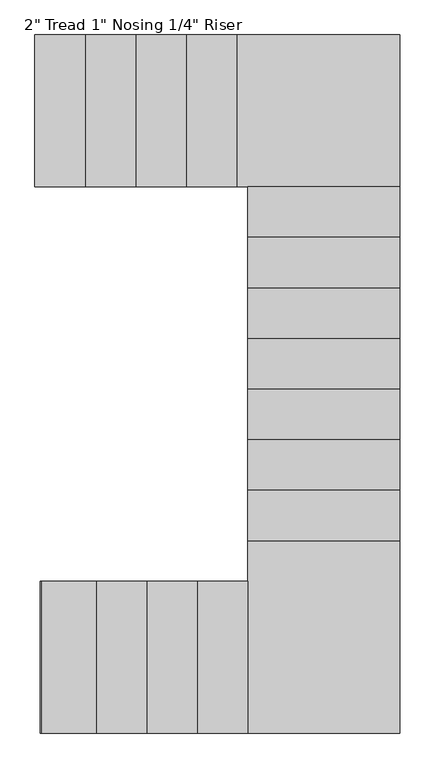
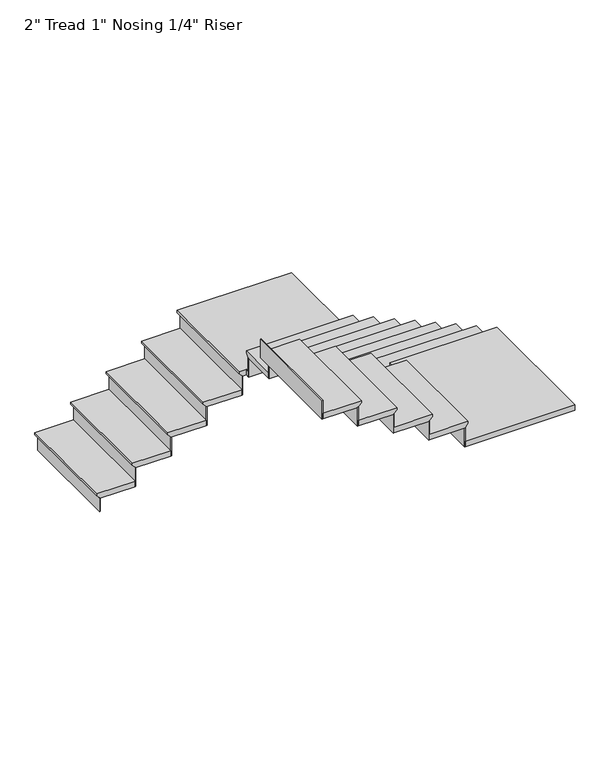
"""IFC4 building model written with IfcOpenShell, lengths in millimetres: stair flight geometry."""

from ifc_helpers import new_model, si_unit, origin, place, context, project, spatial, faceted_brep, source, transform, mapped, element, save


def stair_flight_4d0103da(model_context):
    return source(origin(), model_context, "Body", "Brep", [
        faceted_brep([(-11350.6229553, 1140.6964313, 455.0833333), (-11350.6229553, 1140.6964313, 474.1333333), (-11350.6229553, 2055.0964313, 474.1333333), (-11350.6229553, 2055.0964313, 455.0833333), (-11325.2229553, 1140.6964313, 429.6833333), (-11325.2229553, 2055.0964313, 429.6833333), (-11020.4229553, 1140.6964313, 474.1333333), (-11020.4229553, 2055.0964313, 474.1333333), (-11325.2229553, 2055.0964313, 423.3333333), (-11020.4229553, 2055.0964313, 423.3333333), (-11020.4229553, 1140.6964313, 423.3333333), (-11325.2229553, 1140.6964313, 423.3333333)], [[[0, 1, 2, 3]], [[4, 0, 3, 5]], [[2, 1, 6, 7]], [[8, 9, 10, 11]], [[2, 7, 9, 8, 5, 3]], [[8, 11, 4, 5]], [[6, 1, 0, 4, 11, 10]], [[7, 6, 10, 9]]]),
        faceted_brep([(-11325.2229553, 1140.6964313, 423.3333333), (-11325.2229553, 1140.6964313, 304.8), (-11318.8729553, 1140.6964313, 304.8), (-11318.8729553, 1140.6964313, 423.3333333), (-11325.2229553, 2055.0964313, 423.3333333), (-11318.8729553, 2055.0964313, 423.3333333), (-11318.8729553, 2055.0964313, 304.8), (-11325.2229553, 2055.0964313, 304.8)], [[[0, 1, 2, 3]], [[4, 5, 6, 7]], [[1, 0, 4, 7]], [[2, 1, 7, 6]], [[3, 2, 6, 5]], [[0, 3, 5, 4]]]),
        faceted_brep([(-11020.4229553, 1140.6964313, 592.6666667), (-11020.4229553, 1140.6964313, 423.3333333), (-11014.0729553, 1140.6964313, 423.3333333), (-11014.0729553, 1140.6964313, 592.6666667), (-11020.4229553, 2055.0964313, 592.6666667), (-11014.0729553, 2055.0964313, 592.6666667), (-11014.0729553, 2055.0964313, 423.3333333), (-11020.4229553, 2055.0964313, 423.3333333)], [[[0, 1, 2, 3]], [[4, 5, 6, 7]], [[1, 0, 4, 7]], [[2, 1, 7, 6]], [[3, 2, 6, 5]], [[0, 3, 5, 4]]]),
        faceted_brep([(-11045.8229553, 2055.0964313, 643.4666667), (-11045.8229553, 1140.6964313, 643.4666667), (-10715.6229553, 1140.6964313, 643.4666667), (-10715.6229553, 2055.0964313, 643.4666667), (-11020.4229553, 2055.0964313, 592.6666667), (-10715.6229553, 2055.0964313, 592.6666667), (-10715.6229553, 1140.6964313, 592.6666667), (-11020.4229553, 1140.6964313, 592.6666667), (-11020.4229553, 2055.0964313, 599.0166667), (-11045.8229553, 2055.0964313, 624.4166667), (-11020.4229553, 1140.6964313, 599.0166667), (-11045.8229553, 1140.6964313, 624.4166667)], [[[0, 1, 2, 3]], [[4, 5, 6, 7]], [[0, 3, 5, 4, 8, 9]], [[4, 7, 10, 8]], [[2, 1, 11, 10, 7, 6]], [[3, 2, 6, 5]], [[11, 1, 0, 9]], [[10, 11, 9, 8]]]),
        faceted_brep([(-10715.6229553, 1140.6964313, 762.0), (-10715.6229553, 1140.6964313, 592.6666667), (-10709.2729553, 1140.6964313, 592.6666667), (-10709.2729553, 1140.6964313, 762.0), (-10715.6229553, 2055.0964313, 762.0), (-10709.2729553, 2055.0964313, 762.0), (-10709.2729553, 2055.0964313, 592.6666667), (-10715.6229553, 2055.0964313, 592.6666667)], [[[0, 1, 2, 3]], [[4, 5, 6, 7]], [[1, 0, 4, 7]], [[2, 1, 7, 6]], [[3, 2, 6, 5]], [[0, 3, 5, 4]]]),
        faceted_brep([(-10741.0229553, 2055.0964313, 812.8), (-10741.0229553, 1140.6964313, 812.8), (-10410.8229553, 1140.6964313, 812.8), (-10410.8229553, 2055.0964313, 812.8), (-10715.6229553, 2055.0964313, 762.0), (-10410.8229553, 2055.0964313, 762.0), (-10410.8229553, 1140.6964313, 762.0), (-10715.6229553, 1140.6964313, 762.0), (-10715.6229553, 2055.0964313, 768.35), (-10741.0229553, 2055.0964313, 793.75), (-10715.6229553, 1140.6964313, 768.35), (-10741.0229553, 1140.6964313, 793.75)], [[[0, 1, 2, 3]], [[4, 5, 6, 7]], [[0, 3, 5, 4, 8, 9]], [[4, 7, 10, 8]], [[2, 1, 11, 10, 7, 6]], [[3, 2, 6, 5]], [[11, 1, 0, 9]], [[10, 11, 9, 8]]]),
        faceted_brep([(-10410.8229553, 1140.6964313, 931.3333333), (-10410.8229553, 1140.6964313, 762.0), (-10404.4729553, 1140.6964313, 762.0), (-10404.4729553, 1140.6964313, 931.3333333), (-10410.8229553, 2055.0964313, 931.3333333), (-10404.4729553, 2055.0964313, 931.3333333), (-10404.4729553, 2055.0964313, 762.0), (-10410.8229553, 2055.0964313, 762.0)], [[[0, 1, 2, 3]], [[4, 5, 6, 7]], [[1, 0, 4, 7]], [[2, 1, 7, 6]], [[3, 2, 6, 5]], [[0, 3, 5, 4]]]),
        faceted_brep([(-10436.2229553, 2055.0964313, 982.1333333), (-10436.2229553, 1140.6964313, 982.1333333), (-10106.0229553, 1140.6964313, 982.1333333), (-10106.0229553, 2055.0964313, 982.1333333), (-10410.8229553, 2055.0964313, 931.3333333), (-10106.0229553, 2055.0964313, 931.3333333), (-10106.0229553, 1140.6964313, 931.3333333), (-10410.8229553, 1140.6964313, 931.3333333), (-10410.8229553, 2055.0964313, 937.6833333), (-10436.2229553, 2055.0964313, 963.0833333), (-10410.8229553, 1140.6964313, 937.6833333), (-10436.2229553, 1140.6964313, 963.0833333)], [[[0, 1, 2, 3]], [[4, 5, 6, 7]], [[0, 3, 5, 4, 8, 9]], [[4, 7, 10, 8]], [[2, 1, 11, 10, 7, 6]], [[3, 2, 6, 5]], [[11, 1, 0, 9]], [[10, 11, 9, 8]]]),
        faceted_brep([(-10106.0229553, 1140.6964313, 1100.6666667), (-10106.0229553, 1140.6964313, 931.3333333), (-10099.6729553, 1140.6964313, 931.3333333), (-10099.6729553, 1140.6964313, 1100.6666667), (-10106.0229553, 2055.0964313, 1100.6666667), (-10099.6729553, 2055.0964313, 1100.6666667), (-10099.6729553, 2055.0964313, 931.3333333), (-10106.0229553, 2055.0964313, 931.3333333)], [[[0, 1, 2, 3]], [[4, 5, 6, 7]], [[1, 0, 4, 7]], [[2, 1, 7, 6]], [[3, 2, 6, 5]], [[0, 3, 5, 4]]]),
        faceted_brep([(-9153.5229553, 1115.2964313, 1151.4666667), (-9153.5229553, 2055.0964313, 1151.4666667), (-10131.4229553, 2055.0964313, 1151.4666667), (-10131.4229553, 1140.6964313, 1151.4666667), (-10067.9229553, 1140.6964313, 1151.4666667), (-10067.9229553, 1115.2964313, 1151.4666667), (-9153.5229553, 2055.0964313, 1100.6666667), (-9153.5229553, 1115.2964313, 1100.6666667), (-10067.9229553, 1115.2964313, 1100.6666667), (-10067.9229553, 1140.6964313, 1100.6666667), (-10106.0229553, 1140.6964313, 1100.6666667), (-10106.0229553, 2055.0964313, 1100.6666667), (-10106.0229553, 2055.0964313, 1107.0166667), (-10131.4229553, 2055.0964313, 1132.4166667), (-10106.0229553, 1140.6964313, 1107.0166667), (-10131.4229553, 1140.6964313, 1132.4166667)], [[[0, 1, 2, 3, 4, 5]], [[6, 7, 8, 9, 10, 11]], [[1, 0, 7, 6]], [[2, 1, 6, 11, 12, 13]], [[11, 10, 14, 12]], [[4, 3, 15, 14, 10, 9]], [[5, 4, 9, 8]], [[0, 5, 8, 7]], [[15, 3, 2, 13]], [[14, 15, 13, 12]]]),
        faceted_brep([(-10067.9229553, 1115.2964313, 1270.0), (-10067.9229553, 1115.2964313, 1100.6666667), (-10067.9229553, 1108.9464313, 1100.6666667), (-10067.9229553, 1108.9464313, 1270.0), (-9153.5229553, 1115.2964313, 1270.0), (-9153.5229553, 1108.9464313, 1270.0), (-9153.5229553, 1108.9464313, 1100.6666667), (-9153.5229553, 1115.2964313, 1100.6666667)], [[[0, 1, 2, 3]], [[4, 5, 6, 7]], [[1, 0, 4, 7]], [[2, 1, 7, 6]], [[3, 2, 6, 5]], [[0, 3, 5, 4]]]),
        faceted_brep([(-9153.5229553, 1140.6964313, 1320.8), (-10067.9229553, 1140.6964313, 1320.8), (-10067.9229553, 810.4964313, 1320.8), (-9153.5229553, 810.4964313, 1320.8), (-9153.5229553, 1115.2964313, 1270.0), (-9153.5229553, 810.4964313, 1270.0), (-10067.9229553, 810.4964313, 1270.0), (-10067.9229553, 1115.2964313, 1270.0), (-9153.5229553, 1115.2964313, 1276.35), (-9153.5229553, 1140.6964313, 1301.75), (-10067.9229553, 1115.2964313, 1276.35), (-10067.9229553, 1140.6964313, 1301.75)], [[[0, 1, 2, 3]], [[4, 5, 6, 7]], [[0, 3, 5, 4, 8, 9]], [[4, 7, 10, 8]], [[2, 1, 11, 10, 7, 6]], [[3, 2, 6, 5]], [[11, 1, 0, 9]], [[10, 11, 9, 8]]]),
        faceted_brep([(-10067.9229553, 810.4964313, 1439.3333333), (-10067.9229553, 810.4964313, 1270.0), (-10067.9229553, 804.1464313, 1270.0), (-10067.9229553, 804.1464313, 1439.3333333), (-9153.5229553, 810.4964313, 1439.3333333), (-9153.5229553, 804.1464313, 1439.3333333), (-9153.5229553, 804.1464313, 1270.0), (-9153.5229553, 810.4964313, 1270.0)], [[[0, 1, 2, 3]], [[4, 5, 6, 7]], [[1, 0, 4, 7]], [[2, 1, 7, 6]], [[3, 2, 6, 5]], [[0, 3, 5, 4]]]),
        faceted_brep([(-9153.5229553, 835.8964313, 1490.1333333), (-10067.9229553, 835.8964313, 1490.1333333), (-10067.9229553, 505.6964313, 1490.1333333), (-9153.5229553, 505.6964313, 1490.1333333), (-9153.5229553, 810.4964313, 1439.3333333), (-9153.5229553, 505.6964313, 1439.3333333), (-10067.9229553, 505.6964313, 1439.3333333), (-10067.9229553, 810.4964313, 1439.3333333), (-9153.5229553, 810.4964313, 1445.6833333), (-9153.5229553, 835.8964313, 1471.0833333), (-10067.9229553, 810.4964313, 1445.6833333), (-10067.9229553, 835.8964313, 1471.0833333)], [[[0, 1, 2, 3]], [[4, 5, 6, 7]], [[0, 3, 5, 4, 8, 9]], [[4, 7, 10, 8]], [[2, 1, 11, 10, 7, 6]], [[3, 2, 6, 5]], [[11, 1, 0, 9]], [[10, 11, 9, 8]]]),
        faceted_brep([(-10067.9229553, 505.6964313, 1608.6666667), (-10067.9229553, 505.6964313, 1439.3333333), (-10067.9229553, 499.3464313, 1439.3333333), (-10067.9229553, 499.3464313, 1608.6666667), (-9153.5229553, 505.6964313, 1608.6666667), (-9153.5229553, 499.3464313, 1608.6666667), (-9153.5229553, 499.3464313, 1439.3333333), (-9153.5229553, 505.6964313, 1439.3333333)], [[[0, 1, 2, 3]], [[4, 5, 6, 7]], [[1, 0, 4, 7]], [[2, 1, 7, 6]], [[3, 2, 6, 5]], [[0, 3, 5, 4]]]),
        faceted_brep([(-9153.5229553, 531.0964313, 1659.4666667), (-10067.9229553, 531.0964313, 1659.4666667), (-10067.9229553, 200.8964313, 1659.4666667), (-9153.5229553, 200.8964313, 1659.4666667), (-9153.5229553, 505.6964313, 1608.6666667), (-9153.5229553, 200.8964313, 1608.6666667), (-10067.9229553, 200.8964313, 1608.6666667), (-10067.9229553, 505.6964313, 1608.6666667), (-9153.5229553, 505.6964313, 1615.0166667), (-9153.5229553, 531.0964313, 1640.4166667), (-10067.9229553, 505.6964313, 1615.0166667), (-10067.9229553, 531.0964313, 1640.4166667)], [[[0, 1, 2, 3]], [[4, 5, 6, 7]], [[0, 3, 5, 4, 8, 9]], [[4, 7, 10, 8]], [[2, 1, 11, 10, 7, 6]], [[3, 2, 6, 5]], [[11, 1, 0, 9]], [[10, 11, 9, 8]]]),
        faceted_brep([(-10067.9229553, 200.8964313, 1778.0), (-10067.9229553, 200.8964313, 1608.6666667), (-10067.9229553, 194.5464313, 1608.6666667), (-10067.9229553, 194.5464313, 1778.0), (-9153.5229553, 200.8964313, 1778.0), (-9153.5229553, 194.5464313, 1778.0), (-9153.5229553, 194.5464313, 1608.6666667), (-9153.5229553, 200.8964313, 1608.6666667)], [[[0, 1, 2, 3]], [[4, 5, 6, 7]], [[1, 0, 4, 7]], [[2, 1, 7, 6]], [[3, 2, 6, 5]], [[0, 3, 5, 4]]]),
        faceted_brep([(-9153.5229553, 226.2964313, 1828.8), (-10067.9229553, 226.2964313, 1828.8), (-10067.9229553, -103.9035687, 1828.8), (-9153.5229553, -103.9035687, 1828.8), (-9153.5229553, 200.8964313, 1778.0), (-9153.5229553, -103.9035687, 1778.0), (-10067.9229553, -103.9035687, 1778.0), (-10067.9229553, 200.8964313, 1778.0), (-9153.5229553, 200.8964313, 1784.35), (-9153.5229553, 226.2964313, 1809.75), (-10067.9229553, 200.8964313, 1784.35), (-10067.9229553, 226.2964313, 1809.75)], [[[0, 1, 2, 3]], [[4, 5, 6, 7]], [[0, 3, 5, 4, 8, 9]], [[4, 7, 10, 8]], [[2, 1, 11, 10, 7, 6]], [[3, 2, 6, 5]], [[11, 1, 0, 9]], [[10, 11, 9, 8]]]),
        faceted_brep([(-10067.9229553, -103.9035687, 1947.3333333), (-10067.9229553, -103.9035687, 1778.0), (-10067.9229553, -110.2535687, 1778.0), (-10067.9229553, -110.2535687, 1947.3333333), (-9153.5229553, -103.9035687, 1947.3333333), (-9153.5229553, -110.2535687, 1947.3333333), (-9153.5229553, -110.2535687, 1778.0), (-9153.5229553, -103.9035687, 1778.0)], [[[0, 1, 2, 3]], [[4, 5, 6, 7]], [[1, 0, 4, 7]], [[2, 1, 7, 6]], [[3, 2, 6, 5]], [[0, 3, 5, 4]]]),
        faceted_brep([(-9153.5229553, -78.5035687, 1998.1333333), (-10067.9229553, -78.5035687, 1998.1333333), (-10067.9229553, -408.7035687, 1998.1333333), (-9153.5229553, -408.7035687, 1998.1333333), (-9153.5229553, -103.9035687, 1947.3333333), (-9153.5229553, -408.7035687, 1947.3333333), (-10067.9229553, -408.7035687, 1947.3333333), (-10067.9229553, -103.9035687, 1947.3333333), (-9153.5229553, -103.9035687, 1953.6833333), (-9153.5229553, -78.5035687, 1979.0833333), (-10067.9229553, -103.9035687, 1953.6833333), (-10067.9229553, -78.5035687, 1979.0833333)], [[[0, 1, 2, 3]], [[4, 5, 6, 7]], [[0, 3, 5, 4, 8, 9]], [[4, 7, 10, 8]], [[2, 1, 11, 10, 7, 6]], [[3, 2, 6, 5]], [[11, 1, 0, 9]], [[10, 11, 9, 8]]]),
        faceted_brep([(-10067.9229553, -408.7035687, 2116.6666667), (-10067.9229553, -408.7035687, 1947.3333333), (-10067.9229553, -415.0535687, 1947.3333333), (-10067.9229553, -415.0535687, 2116.6666667), (-9153.5229553, -408.7035687, 2116.6666667), (-9153.5229553, -415.0535687, 2116.6666667), (-9153.5229553, -415.0535687, 1947.3333333), (-9153.5229553, -408.7035687, 1947.3333333)], [[[0, 1, 2, 3]], [[4, 5, 6, 7]], [[1, 0, 4, 7]], [[2, 1, 7, 6]], [[3, 2, 6, 5]], [[0, 3, 5, 4]]]),
        faceted_brep([(-9153.5229553, -383.3035687, 2167.4666667), (-10067.9229553, -383.3035687, 2167.4666667), (-10067.9229553, -713.5035687, 2167.4666667), (-9153.5229553, -713.5035687, 2167.4666667), (-9153.5229553, -408.7035687, 2116.6666667), (-9153.5229553, -713.5035687, 2116.6666667), (-10067.9229553, -713.5035687, 2116.6666667), (-10067.9229553, -408.7035687, 2116.6666667), (-9153.5229553, -408.7035687, 2123.0166667), (-9153.5229553, -383.3035687, 2148.4166667), (-10067.9229553, -408.7035687, 2123.0166667), (-10067.9229553, -383.3035687, 2148.4166667)], [[[0, 1, 2, 3]], [[4, 5, 6, 7]], [[0, 3, 5, 4, 8, 9]], [[4, 7, 10, 8]], [[2, 1, 11, 10, 7, 6]], [[3, 2, 6, 5]], [[11, 1, 0, 9]], [[10, 11, 9, 8]]]),
        faceted_brep([(-10067.9229553, -713.5035687, 2286.0), (-10067.9229553, -713.5035687, 2116.6666667), (-10067.9229553, -719.8535687, 2116.6666667), (-10067.9229553, -719.8535687, 2286.0), (-9153.5229553, -713.5035687, 2286.0), (-9153.5229553, -719.8535687, 2286.0), (-9153.5229553, -719.8535687, 2116.6666667), (-9153.5229553, -713.5035687, 2116.6666667)], [[[0, 1, 2, 3]], [[4, 5, 6, 7]], [[1, 0, 4, 7]], [[2, 1, 7, 6]], [[3, 2, 6, 5]], [[0, 3, 5, 4]]]),
        faceted_brep([(-9153.5229553, -688.1035687, 2336.8), (-10067.9229553, -688.1035687, 2336.8), (-10067.9229553, -1018.3035687, 2336.8), (-9153.5229553, -1018.3035687, 2336.8), (-9153.5229553, -713.5035687, 2286.0), (-9153.5229553, -1018.3035687, 2286.0), (-10067.9229553, -1018.3035687, 2286.0), (-10067.9229553, -713.5035687, 2286.0), (-9153.5229553, -713.5035687, 2292.35), (-9153.5229553, -688.1035687, 2317.75), (-10067.9229553, -713.5035687, 2292.35), (-10067.9229553, -688.1035687, 2317.75)], [[[0, 1, 2, 3]], [[4, 5, 6, 7]], [[0, 3, 5, 4, 8, 9]], [[4, 7, 10, 8]], [[2, 1, 11, 10, 7, 6]], [[3, 2, 6, 5]], [[11, 1, 0, 9]], [[10, 11, 9, 8]]]),
        faceted_brep([(-10067.9229553, -1018.3035687, 2455.3333333), (-10067.9229553, -1018.3035687, 2286.0), (-10067.9229553, -1024.6535687, 2286.0), (-10067.9229553, -1024.6535687, 2455.3333333), (-9153.5229553, -1018.3035687, 2455.3333333), (-9153.5229553, -1024.6535687, 2455.3333333), (-9153.5229553, -1024.6535687, 2286.0), (-9153.5229553, -1018.3035687, 2286.0)], [[[0, 1, 2, 3]], [[4, 5, 6, 7]], [[1, 0, 4, 7]], [[2, 1, 7, 6]], [[3, 2, 6, 5]], [[0, 3, 5, 4]]]),
        faceted_brep([(-10093.3229553, -2148.6035687, 2506.1333333), (-9153.5229553, -2148.6035687, 2506.1333333), (-9153.5229553, -992.9035687, 2506.1333333), (-10067.9229553, -992.9035687, 2506.1333333), (-10067.9229553, -1234.2035687, 2506.1333333), (-10093.3229553, -1234.2035687, 2506.1333333), (-9153.5229553, -2148.6035687, 2455.3333333), (-10093.3229553, -2148.6035687, 2455.3333333), (-10093.3229553, -1234.2035687, 2455.3333333), (-10067.9229553, -1234.2035687, 2455.3333333), (-10067.9229553, -1018.3035687, 2455.3333333), (-9153.5229553, -1018.3035687, 2455.3333333), (-9153.5229553, -1018.3035687, 2461.6833333), (-9153.5229553, -992.9035687, 2487.0833333), (-10067.9229553, -1018.3035687, 2461.6833333), (-10067.9229553, -992.9035687, 2487.0833333)], [[[0, 1, 2, 3, 4, 5]], [[6, 7, 8, 9, 10, 11]], [[1, 0, 7, 6]], [[2, 1, 6, 11, 12, 13]], [[11, 10, 14, 12]], [[4, 3, 15, 14, 10, 9]], [[5, 4, 9, 8]], [[0, 5, 8, 7]], [[15, 3, 2, 13]], [[14, 15, 13, 12]]]),
        faceted_brep([(-10093.3229553, -1234.2035687, 2624.6666667), (-10093.3229553, -1234.2035687, 2455.3333333), (-10099.6729553, -1234.2035687, 2455.3333333), (-10099.6729553, -1234.2035687, 2624.6666667), (-10093.3229553, -2148.6035687, 2624.6666667), (-10099.6729553, -2148.6035687, 2624.6666667), (-10099.6729553, -2148.6035687, 2455.3333333), (-10093.3229553, -2148.6035687, 2455.3333333)], [[[0, 1, 2, 3]], [[4, 5, 6, 7]], [[1, 0, 4, 7]], [[2, 1, 7, 6]], [[3, 2, 6, 5]], [[0, 3, 5, 4]]]),
        faceted_brep([(-10067.9229553, -2148.6035687, 2675.4666667), (-10067.9229553, -1234.2035687, 2675.4666667), (-10398.1229553, -1234.2035687, 2675.4666667), (-10398.1229553, -2148.6035687, 2675.4666667), (-10093.3229553, -2148.6035687, 2624.6666667), (-10398.1229553, -2148.6035687, 2624.6666667), (-10398.1229553, -1234.2035687, 2624.6666667), (-10093.3229553, -1234.2035687, 2624.6666667), (-10093.3229553, -2148.6035687, 2631.0166667), (-10067.9229553, -2148.6035687, 2656.4166667), (-10093.3229553, -1234.2035687, 2631.0166667), (-10067.9229553, -1234.2035687, 2656.4166667)], [[[0, 1, 2, 3]], [[4, 5, 6, 7]], [[0, 3, 5, 4, 8, 9]], [[4, 7, 10, 8]], [[2, 1, 11, 10, 7, 6]], [[3, 2, 6, 5]], [[11, 1, 0, 9]], [[10, 11, 9, 8]]]),
        faceted_brep([(-10398.1229553, -1234.2035687, 2794.0), (-10398.1229553, -1234.2035687, 2624.6666667), (-10404.4729553, -1234.2035687, 2624.6666667), (-10404.4729553, -1234.2035687, 2794.0), (-10398.1229553, -2148.6035687, 2794.0), (-10404.4729553, -2148.6035687, 2794.0), (-10404.4729553, -2148.6035687, 2624.6666667), (-10398.1229553, -2148.6035687, 2624.6666667)], [[[0, 1, 2, 3]], [[4, 5, 6, 7]], [[1, 0, 4, 7]], [[2, 1, 7, 6]], [[3, 2, 6, 5]], [[0, 3, 5, 4]]]),
        faceted_brep([(-10372.7229553, -2148.6035687, 2844.8), (-10372.7229553, -1234.2035687, 2844.8), (-10702.9229553, -1234.2035687, 2844.8), (-10702.9229553, -2148.6035687, 2844.8), (-10398.1229553, -2148.6035687, 2794.0), (-10702.9229553, -2148.6035687, 2794.0), (-10702.9229553, -1234.2035687, 2794.0), (-10398.1229553, -1234.2035687, 2794.0), (-10398.1229553, -2148.6035687, 2800.35), (-10372.7229553, -2148.6035687, 2825.75), (-10398.1229553, -1234.2035687, 2800.35), (-10372.7229553, -1234.2035687, 2825.75)], [[[0, 1, 2, 3]], [[4, 5, 6, 7]], [[0, 3, 5, 4, 8, 9]], [[4, 7, 10, 8]], [[2, 1, 11, 10, 7, 6]], [[3, 2, 6, 5]], [[11, 1, 0, 9]], [[10, 11, 9, 8]]]),
        faceted_brep([(-10702.9229553, -1234.2035687, 2963.3333333), (-10702.9229553, -1234.2035687, 2794.0), (-10709.2729553, -1234.2035687, 2794.0), (-10709.2729553, -1234.2035687, 2963.3333333), (-10702.9229553, -2148.6035687, 2963.3333333), (-10709.2729553, -2148.6035687, 2963.3333333), (-10709.2729553, -2148.6035687, 2794.0), (-10702.9229553, -2148.6035687, 2794.0)], [[[0, 1, 2, 3]], [[4, 5, 6, 7]], [[1, 0, 4, 7]], [[2, 1, 7, 6]], [[3, 2, 6, 5]], [[0, 3, 5, 4]]]),
        faceted_brep([(-10677.5229553, -2148.6035687, 3014.1333333), (-10677.5229553, -1234.2035687, 3014.1333333), (-11007.7229553, -1234.2035687, 3014.1333333), (-11007.7229553, -2148.6035687, 3014.1333333), (-10702.9229553, -2148.6035687, 2963.3333333), (-11007.7229553, -2148.6035687, 2963.3333333), (-11007.7229553, -1234.2035687, 2963.3333333), (-10702.9229553, -1234.2035687, 2963.3333333), (-10702.9229553, -2148.6035687, 2969.6833333), (-10677.5229553, -2148.6035687, 2995.0833333), (-10702.9229553, -1234.2035687, 2969.6833333), (-10677.5229553, -1234.2035687, 2995.0833333)], [[[0, 1, 2, 3]], [[4, 5, 6, 7]], [[0, 3, 5, 4, 8, 9]], [[4, 7, 10, 8]], [[2, 1, 11, 10, 7, 6]], [[3, 2, 6, 5]], [[11, 1, 0, 9]], [[10, 11, 9, 8]]]),
        faceted_brep([(-11007.7229553, -1234.2035687, 3132.6666667), (-11007.7229553, -1234.2035687, 2963.3333333), (-11014.0729553, -1234.2035687, 2963.3333333), (-11014.0729553, -1234.2035687, 3132.6666667), (-11007.7229553, -2148.6035687, 3132.6666667), (-11014.0729553, -2148.6035687, 3132.6666667), (-11014.0729553, -2148.6035687, 2963.3333333), (-11007.7229553, -2148.6035687, 2963.3333333)], [[[0, 1, 2, 3]], [[4, 5, 6, 7]], [[1, 0, 4, 7]], [[2, 1, 7, 6]], [[3, 2, 6, 5]], [[0, 3, 5, 4]]]),
        faceted_brep([(-11312.5229553, -1234.2035687, 3302.0), (-11312.5229553, -1234.2035687, 3132.6666667), (-11318.8729553, -1234.2035687, 3132.6666667), (-11318.8729553, -1234.2035687, 3302.0), (-11312.5229553, -2148.6035687, 3302.0), (-11318.8729553, -2148.6035687, 3302.0), (-11318.8729553, -2148.6035687, 3132.6666667), (-11312.5229553, -2148.6035687, 3132.6666667)], [[[0, 1, 2, 3]], [[4, 5, 6, 7]], [[1, 0, 4, 7]], [[2, 1, 7, 6]], [[3, 2, 6, 5]], [[0, 3, 5, 4]]]),
        faceted_brep([(-10982.3229553, -2148.6035687, 3183.4666667), (-10982.3229553, -1234.2035687, 3183.4666667), (-11312.5229553, -1234.2035687, 3183.4666667), (-11312.5229553, -2148.6035687, 3183.4666667), (-11007.7229553, -2148.6035687, 3132.6666667), (-11312.5229553, -2148.6035687, 3132.6666667), (-11312.5229553, -1234.2035687, 3132.6666667), (-11007.7229553, -1234.2035687, 3132.6666667), (-11007.7229553, -2148.6035687, 3139.0166667), (-10982.3229553, -2148.6035687, 3164.4166667), (-11007.7229553, -1234.2035687, 3139.0166667), (-10982.3229553, -1234.2035687, 3164.4166667)], [[[0, 1, 2, 3]], [[4, 5, 6, 7]], [[0, 3, 5, 4, 8, 9]], [[4, 7, 10, 8]], [[2, 1, 11, 10, 7, 6]], [[3, 2, 6, 5]], [[11, 1, 0, 9]], [[10, 11, 9, 8]]]),
    ])


if __name__ == "__main__":
    model = new_model("IFC4")
    model_context = context("Model", 3, world=origin())
    ifc_project = project(units=[si_unit("LENGTHUNIT", "METRE", prefix="MILLI")], contexts=[model_context])
    site = spatial("IfcSite", under=ifc_project)
    building = spatial("IfcBuilding", under=site)
    placement = place(None, origin())
    stair_flight_shape = stair_flight_4d0103da(model_context)
    element("IfcStairFlight", 1, ObjectType="2\" Tread 1\" Nosing 1/4\" Riser", at=placement, inside=building, context=model_context, shape_type="MappedRepresentation", body=[
        mapped(stair_flight_shape, transform((0.0, 0.0, 0.0), x_axis=(1.0, 0.0, 0.0), y_axis=(0.0, 1.0, 0.0), z_axis=(0.0, 0.0, 1.0))),
    ])
    save(model, "model.ifc")
